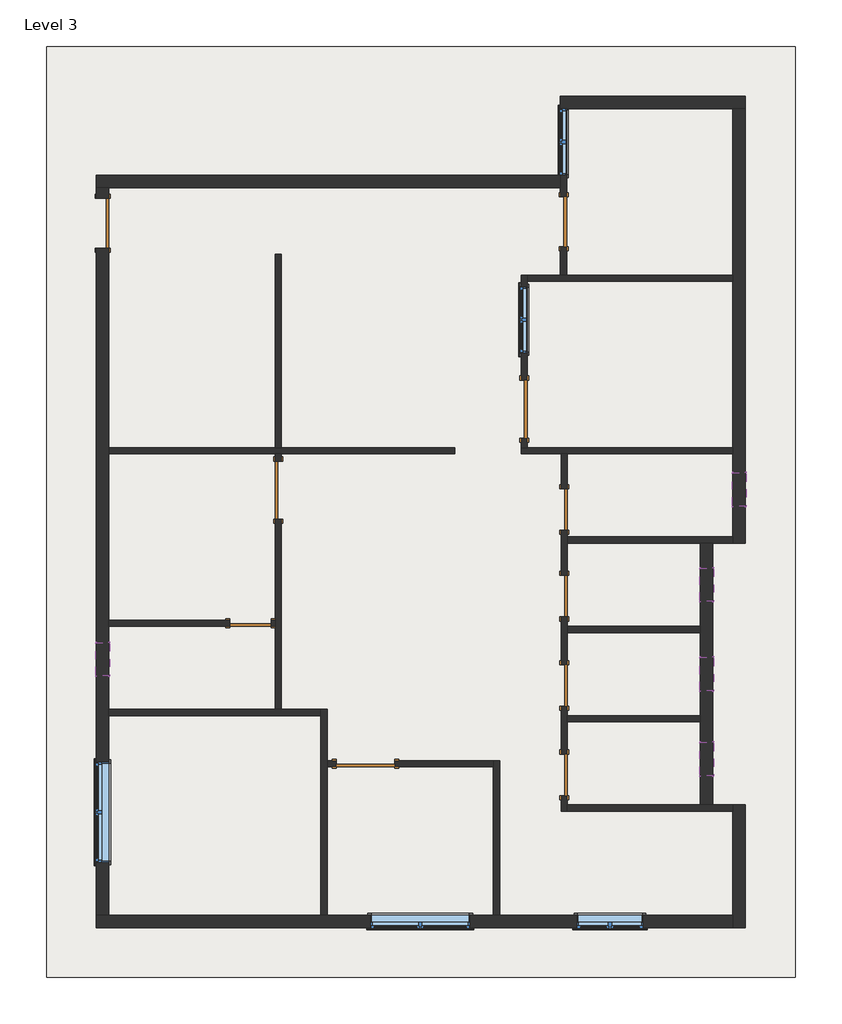
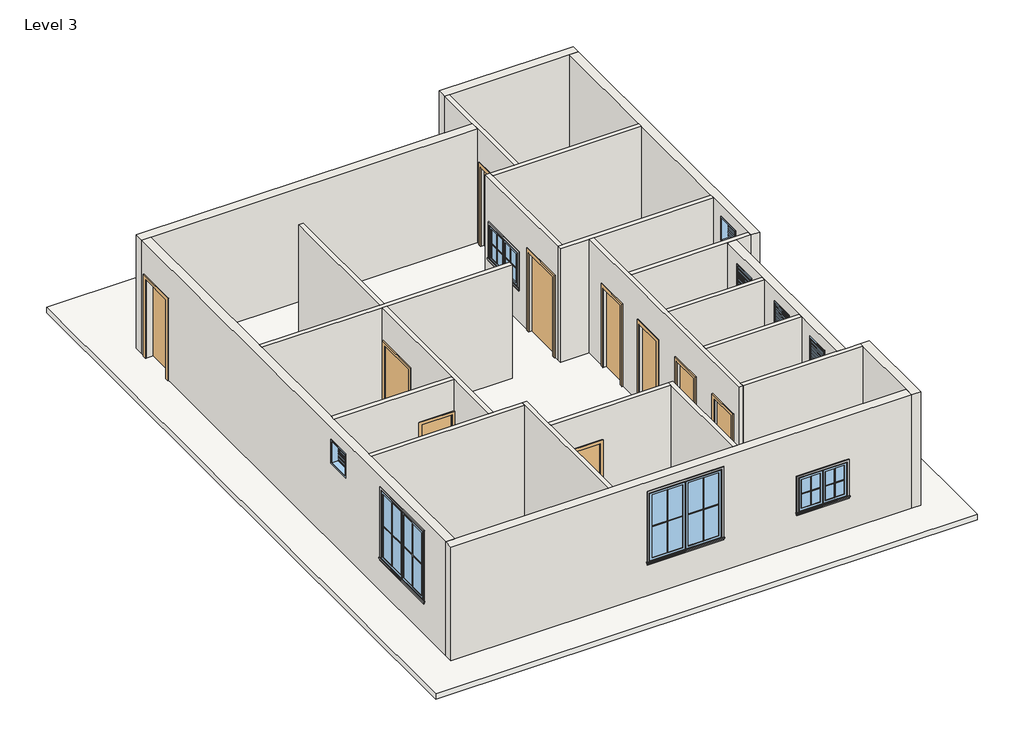
# One storey, incomplete: 23 walls, 20 proxies, 10 doors, 10 windows, 1 roof.
# Revit data of these elements (continued)
# Elements 48, 49, 50, 51, 52, 53, 54 (IfcWall, "WALL 9\"") (continued)
#   Base Offset = 0' - 0"
#   Unconnected Height = 10' - 0"
#   wall height = 10' - 0"
#   Phase Created = New Construction
#   Base Constraint = Level 3
#   Materials on its faces: "Default Wall", "Wood - Stained"
# Element 55 (IfcWindow, "Window-Casement-Double : WIN 4'")
#   Mark = "23"
#   Window Inset = 0' - 0"
#   Interior Wall Closure = 0' - 2 1/4"
#   Frame Extension = 0' - 0 1/4"
#   Exterior Wall Closure = 0' - 1 1/4"
#   Interior Trim Visibility = yes
#   Exterior Trim Visibility = yes
#   Phase Created = New Construction
#   Materials on its faces: "Wood - Stained", "Glass", "Clad - White"
# Element 56 (IfcWindow, "Window-Casement-Double : WIN 4'")
#   Mark = "24"
#   Window Inset = 0' - 0"
#   Interior Wall Closure = 0' - 2 1/4"
#   Frame Extension = 0' - 0 1/4"
#   Exterior Wall Closure = 0' - 1 1/4"
#   Interior Trim Visibility = yes
#   Exterior Trim Visibility = yes
#   Phase Created = New Construction
#   Materials on its faces: "Wood - Stained", "Glass", "Clad - White"
# Element 57 (IfcWindow, "Window-Casement-Double : WIN 4'")
#   Mark = "25"
#   Window Inset = 0' - 0"
#   Interior Wall Closure = 0' - 2 1/4"
#   Frame Extension = 0' - 0 1/4"
#   Exterior Wall Closure = 0' - 1 1/4"
#   Interior Trim Visibility = yes
#   Exterior Trim Visibility = yes
#   Phase Created = New Construction
#   Materials on its faces: "Wood - Stained", "Glass", "Clad - White"
# Element 58 (IfcWindow, "Window-Casement-Double : WIN 6'")
#   Mark = "21"
#   Window Inset = 0' - 0"
#   Interior Wall Closure = 0' - 2 1/4"
#   Frame Extension = 0' - 0 1/4"
#   Exterior Wall Closure = 0' - 1 1/4"
#   Interior Trim Visibility = yes
#   Exterior Trim Visibility = yes
#   Phase Created = New Construction
#   Materials on its faces: "Wood - Stained", "Glass", "Clad - White"
# Element 59 (IfcWindow, "Window-Casement-Double : WIN 6'")
#   Mark = "22"
#   Window Inset = 0' - 0"
#   Interior Wall Closure = 0' - 2 1/4"
#   Frame Extension = 0' - 0 1/4"
#   Exterior Wall Closure = 0' - 1 1/4"
#   Interior Trim Visibility = yes
#   Exterior Trim Visibility = yes
#   Phase Created = New Construction
#   Materials on its faces: "Wood - Stained", "Glass", "Clad - White"
# Element 60 (IfcWindow, "Window-Louvers : 24\" x 24\"")
#   Mark = "26"
#   Blade Width = 1' - 10 1/2"
#   Phase Created = New Construction
#   Materials on its faces: "Birch"
# Element 61 (IfcWindow, "Window-Louvers : 24\" x 24\"")
#   Mark = "27"
#   Blade Width = 1' - 10 1/2"
#   Phase Created = New Construction
#   Materials on its faces: "Birch"
# Element 62 (IfcWindow, "Window-Louvers : 24\" x 24\"")
#   Mark = "28"
#   Blade Width = 1' - 10 1/2"
#   Phase Created = New Construction
#   Materials on its faces: "Birch"
# Element 63 (IfcWindow, "Window-Louvers : 24\" x 24\"")
#   Mark = "29"
#   Blade Width = 1' - 10 1/2"
#   Phase Created = New Construction
#   Materials on its faces: "Birch"
# Element 64 (IfcWindow, "Window-Louvers : 24\" x 24\"")
#   Mark = "30"
#   Blade Width = 1' - 10 1/2"
#   Phase Created = New Construction
#   Materials on its faces: "Birch"
# Materials
#   "Door - Panel": class "Wood", colour RGB 210 159 95, transparency 0, Cost = 0
#   "Door - Frame": colour RGB 118 70 51, transparency 0, Cost = 0
#   "Wood - Stained": class "Wood", colour RGB 224 178 126, transparency 0, Cost = 0
#   "Glass": class "Glass", colour RGB 0 128 192, transparency 0.75, Description = "Soda Lime Glass", Cost = 0
#   "Clad - White": class "Wood", colour RGB 242 242 238, transparency 0, Cost = 0
#   "Birch": class "Wood", colour RGB 224 178 126, transparency 0, Description = "Betula Alleghaniensis", Cost = 0
#   "Default Roof": colour RGB 88 101 114, transparency 0, Cost = 0
#   "Cherry": class "Wood", colour RGB 226 177 128, transparency 0, Description = "Prunus Serotina", Cost = 0
#   "Wood Planks": class "Wood", colour RGB 193 160 115, transparency 0, Description = "Physical material.", Cost = 0
#   "Default Wall": colour RGB 128 128 128, transparency 0, Cost = 0
